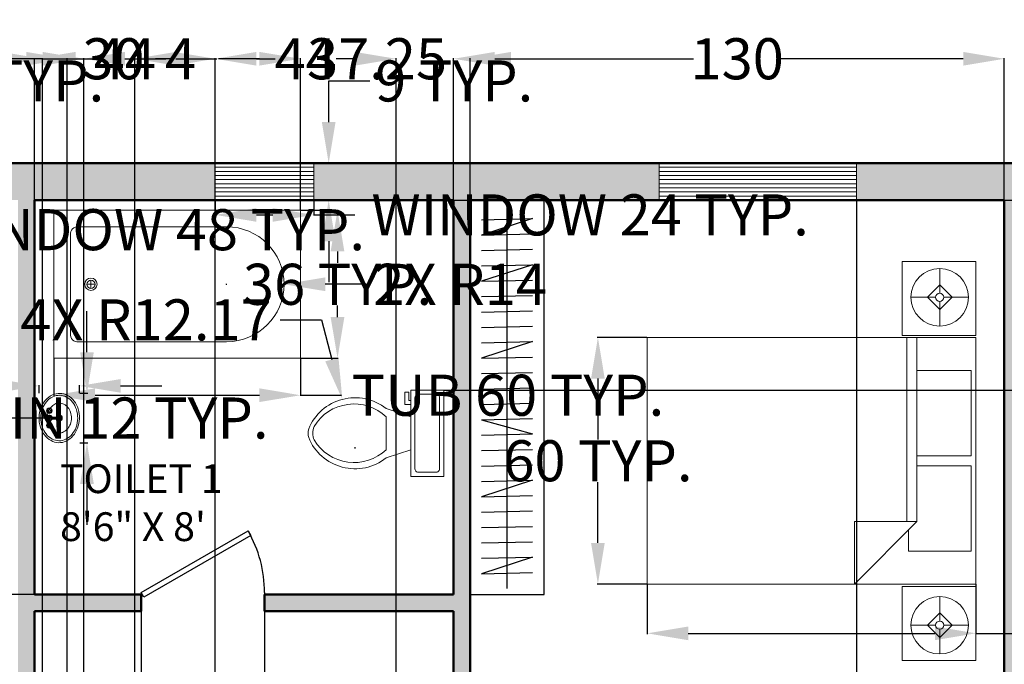
# Model space of a CAD drawing. Units: inches. Extents: x 133 to 758, y -29 to 543.
# Tile 6 of 7: x 386 to 626, y 386 to 543. Entities that reach past the tile are written whole.
import ezdxf

# ---------------------------------------------------------------- set-up
doc = ezdxf.new("R2010")
doc.units = ezdxf.units.IN
doc.header["$MEASUREMENT"] = 0
for name, color, linetype, lineweight in [('A-ANNO-DIMS', 2, 'Continuous', 18), ('A-AREA-IDEN', 7, 'Continuous', 25), ('A-FLOR-CASE', 32, 'Continuous', 25), ('A-FLOR-FIXT', 9, 'Continuous', 20), ('A-FURN', 8, 'Continuous', 18), ('A-WALL', 7, 'Continuous', 50), ('DOOR', 40, 'Continuous', 25), ('WINDOW', 151, 'Continuous', 18)]:
    doc.layers.add(name, color=color, linetype=linetype, lineweight=lineweight)
doc.layers.add('A-WALL-PATT', color=251, linetype='Continuous', lineweight=13, true_color=0x636466)
doc.styles.get("Standard").update_dxf_attribs({"font": 'arial.ttf'})
doc.dimstyles.get("Standard").update_dxf_attribs({"dimtxt": 10, "dimasz": 10, "dimexe": 0.18, "dimexo": 0.0625, "dimgap": 0.09, "dimtad": 0, "dimtih": 1, "dimtoh": 1, "dimdec": 0, "dimzin": 0, "dimdsep": 46, "dimlunit": 4, "dimtxsty": 'Standard', "dimcen": 0.09, "dimadec": 0, "dimazin": 0, "dimtfac": 1, "dimtdec": 0, "dimtofl": 0, "dimtmove": 0, "dimatfit": 3, "dimfxl": 1, "dimtolj": 1, "dimtzin": 0, "dimarcsym": 0})

# ---------------------------------------------------------------- blocks, each defined once
blk = doc.blocks.new('*U11')
for p, q in [((0, 0), (0, -6)), ((40, 0), (40, -6))]:
    blk.add_line(p, q)
blk.add_lwpolyline([(0, 0), (34.64, 20), (35.52, 18.48), (0.87, -1.52)], close=True)
blk.add_arc((0, 0), 40, 0, 30)
blk = doc.blocks.new('Bed - Queen')
for p, q in [((0, -80.00003), (0, 0)), ((0, 0), (59.99999, 0)), ((59.99999, 0), (59.99999, -80.00003)), ((7.99999, -1.2), (28.79998, -1.2)), ((7.99999, -14.4), (7.99999, -1.2)), ((28.79998, -1.2), (28.79998, -14.4)), ((31.19999, -1.2), (51.99999, -1.2)), ((31.19999, -14.4), (31.19999, -1.2)), ((51.99999, -1.2), (51.99999, -16.4)), ((0, -14.4), (44.8, -14.4)), ((59.99999, -29.6), (44.8, -14.4)), ((44.8, -14.4), (44.8, -29.6)), ((51.99999, -16.4), (46.79936, -16.4)), ((44.8, -16.8), (0, -16.8)), ((44.8, -29.6), (59.99999, -29.6)), ((59.99999, -80.00003), (0, -80.00003))]:
    blk.add_line(p, q)
blk = doc.blocks.new('Lamp - Table')
for p, q in [((0, 7), (0, 1)), ((0, 3), (-3, 0)), ((3, 0), (0, 3)), ((-1, 0), (-7, 0)), ((-3, 0), (0, -3)), ((0, -3), (3, 0)), ((1, 0), (7, 0)), ((0, -1), (0, -7))]:
    blk.add_line(p, q)
for radius in [7, 1]:
    blk.add_circle((0, 0), radius)
blk = doc.blocks.new('Bath Tub - 26 x 60 in.')
for p, q in [((8, -18), (10, -18)), ((9, -17), (9, -19))]:
    blk.add_line(p, q)
blk.add_lwpolyline([(0, -36), (0, 0), (60, 0), (60, -36)], close=True)
for points in [[(6, -4), (42, -4)], [(4, -30), (4, -6)], [(42, -32), (6, -32)]]:
    blk.add_lwpolyline(points)
for radius in [1.5, 1]:
    blk.add_circle((9, -18), radius)
for centre, radius, start, end in [((5.75, -5.75), 1.77, 81.8699, 188.1301), ((42, -18), 14, 270, 90), ((5.75, -30.25), 1.77, 171.8699, 278.1301)]:
    blk.add_arc(centre, radius, start, end)
blk = doc.blocks.new('Toilet - top')
for p, q in [((9.5, -6), (9.5, -2)), ((-10, -8.5), (-8, -8.5)), ((-10, -9.5), (-10, -8.5)), ((-7, -9.5), (-10, -9.5)), ((-8, -8.5), (-8, -8)), ((-7, -8), (-7, -9.5)), ((-4, -8), (-6, -14)), ((4, -8), (6, -14)), ((4, -14), (-4, -14))]:
    blk.add_line(p, q)
blk.add_lwpolyline([(10.5, -8), (10.5, 0), (-10.5, 0), (-10.5, -8)], close=True)
for points in [[(-9.5, -2), (-9.5, -6)], [(8.5, -1), (-8.5, -1)], [(-8.5, -7), (8.5, -7)]]:
    blk.add_lwpolyline(points)
for centre, radius, start, end in [((-8.62, -1.88), 0.884, 81.8699, 188.1301), ((8.62, -1.88), 0.884, 351.8699, 98.1301), ((-8.62, -6.12), 0.884, 171.8699, 278.1301), ((8.62, -6.12), 0.884, 261.8699, 8.1301), ((3.52, -21.58), 12.17, 141.4691, 247.9714), ((4.2, -21.82), 11.33, 136.3677, 238.9468), ((-3.52, -21.58), 12.17, 292.0284, 38.5307), ((-4.2, -21.82), 11.33, 301.053, 43.6321), ((0, -27.88), 4, 245.7318, 294.2682), ((0, -29), 4, 254.8605, 285.1395)]:
    blk.add_arc(centre, radius, start, end)
blk = doc.blocks.new('Sink - Oval top')
for p, q in [((-1, 0), (1, 0)), ((0, 1), (0, -1))]:
    blk.add_line(p, q)
for points in [[(-12.23, 0.39, 0.117634), (-11.46, -3.36, 0.104469), (-8.88, -6.8, 0.090016), (-5.08, -9.07, 0.08192), (-0.32, -10.02, 0.08192), (4.49, -9.38, 0.090016), (8.42, -7.36, 0.104469), (11.22, -4.09, 0.117634), (12.23, -0.39, 0.117634), (11.46, 3.36, 0.104469), (8.88, 6.8, 0.090016), (5.08, 9.07, 0.08192), (0.32, 10.02, 0.08192), (-4.49, 9.38, 0.090016), (-8.42, 7.36, 0.104469), (-11.22, 4.09, 0.117634)], [(-11.29, 0.16, 0.118622), (-10.52, -3.25, 0.104678), (-8.07, -6.36, 0.089562), (-4.54, -8.37, 0.081185), (-0.13, -9.15, 0.081185), (4.3, -8.49, 0.089562), (7.89, -6.58, 0.104678), (10.42, -3.55, 0.118622), (11.29, -0.16, 0.118622), (10.52, 3.25, 0.104678), (8.07, 6.36, 0.089562), (4.54, 8.37, 0.081185), (0.13, 9.15, 0.081185), (-4.3, 8.49, 0.089562), (-7.89, 6.58, 0.104678), (-10.42, 3.55, 0.118622)], [(-7.42, 0.08, 0.118283), (-6.91, -2.17, 0.104607), (-5.29, -4.21, 0.089718), (-2.97, -5.53, 0.081436), (-0.07, -6.04, 0.081436), (2.84, -5.59, 0.089718), (5.2, -4.33, 0.104607), (6.86, -2.32, 0.118283), (7.42, -0.08, 0.118283), (6.91, 2.17, 0.104607), (5.29, 4.21, 0.089718), (2.97, 5.53, 0.081436), (0.07, 6.04, 0.081436), (-2.84, 5.59, 0.089718), (-5.2, 4.33, 0.104607), (-6.86, 2.32, 0.118283)]]:
    blk.add_lwpolyline(points, format="xyb", close=True)
for radius in [1.5, 1]:
    blk.add_circle((0, 0), radius)
blk = doc.blocks.new('Faucet - Bathroom top')
for p, q in [((-4.107, 0.125), (-4.375, 0.125)), ((-3.75, 0.4788), (-3.75, 0.75)), ((-3.5, 0.482), (-3.5, 0.75)), ((-3.1461, 0.125), (-2.875, 0.125)), ((3.143, 0.125), (2.875, 0.125)), ((3.5, 0.4788), (3.5, 0.75)), ((3.75, 0.482), (3.75, 0.75)), ((4.1039, 0.125), (4.375, 0.125)), ((-4.1039, -0.125), (-4.375, -0.125)), ((-3.75, -0.4821), (-3.75, -0.75)), ((-3.5, -0.4789), (-3.5, -0.75)), ((-3.143, -0.125), (-2.875, -0.125)), ((-0.5, -0.8639), (-0.5, -4.5)), ((0.5, -4.5), (0.5, -0.8631)), ((3.1461, -0.125), (2.875, -0.125)), ((3.5, -0.4821), (3.5, -0.75)), ((3.75, -0.4789), (3.75, -0.75)), ((4.107, -0.125), (4.375, -0.125))]:
    blk.add_line(p, q)
for centre, radius in [((-3.625, 0), 1.375), ((-4.625, 0), 0.2795), ((-3.625, 0), 0.5), ((-3.625, 1), 0.2795), ((-2.625, 0), 0.2795), ((0, 0), 0.5), ((3.625, 0), 1.375), ((2.625, 0), 0.2795), ((3.625, 0), 0.5), ((3.625, 1), 0.2795), ((4.625, 0), 0.2795), ((-3.625, -1), 0.2795), ((3.625, -1), 0.2795)]:
    blk.add_circle(centre, radius)
for centre, radius, start, end in [((-3.625, 0), 1, 105.2407, 164.2093), ((-3.625, 0), 1, 16.44125, 74.07887), ((0, 0), 1.5, 289.6514, 250.3603), ((0, 0), 1, 300.3431, 239.7554), ((3.625, 0), 1, 106.12, 164.0884), ((3.625, 0), 1, 16.23422, 73.90469), ((-3.625, 0), 1, 196.2342, 253.9047), ((-3.625, 0), 1, 286.12, 344.0884), ((0, -4.5), 0.5, 180, 0), ((3.625, 0), 1, 196.4413, 254.0789), ((3.625, 0), 1, 285.2407, 344.2093)]:
    blk.add_arc(centre, radius, start, end)
blk = doc.blocks.new('WIN-48IN')
for p, q in [((0, 8), (48, 8)), ((0, 7), (48, 7)), ((0, 6), (48, 6)), ((0, 5), (48, 5)), ((0, 4), (48, 4)), ((0, 3), (48, 3)), ((0, 2), (48, 2)), ((0, 1), (48, 1)), ((0, 0), (48, 0))]:
    blk.add_line(p, q)
blk.add_lwpolyline([(48, 9), (48, 0), (0, 0), (0, 9)], close=True)
blk = doc.blocks.new('WIN-24IN')
for p, q in [((0, 8), (24, 8)), ((0, 7), (24, 7)), ((0, 6), (24, 6)), ((0, 5), (24, 5)), ((0, 4), (24, 4)), ((0, 3), (24, 3)), ((0, 2), (24, 2)), ((0, 1), (24, 1))]:
    blk.add_line(p, q)
blk.add_lwpolyline([(24, 9), (24, 0), (0, 0), (0, 9)], close=True)
blk = doc.blocks.new('WARDROBE-96X18IN')
for p, q in [((18, 96), (0, 96)), ((0, 96), (0, 0)), ((18, 0), (18, 96)), ((9, 1.47), (9, 94.4)), ((2.8, 91.24), (15.16, 91.53)), ((15.16, 91.53), (2.8, 87.49)), ((2.8, 87.49), (15.16, 87.78)), ((2.8, 83.75), (15.16, 84.04)), ((2.8, 80), (15.16, 80.29)), ((15.16, 80.29), (2.8, 76.25)), ((2.8, 76.25), (15.16, 76.54)), ((2.8, 72.51), (15.16, 72.8)), ((2.8, 68.76), (15.16, 69.05)), ((2.8, 65.01), (15.16, 65.3)), ((2.8, 61.27), (15.16, 61.56)), ((15.16, 61.56), (2.8, 57.52)), ((2.8, 57.52), (15.16, 57.81)), ((2.8, 53.77), (15.16, 54.06)), ((2.8, 50.03), (15.16, 50.32)), ((2.8, 46.28), (15.16, 46.57)), ((2.8, 42.53), (15.16, 42.82)), ((2.8, 42.53), (15.16, 39.08)), ((2.8, 38.79), (15.16, 39.08)), ((2.8, 35.04), (15.16, 35.33)), ((2.8, 31.29), (15.16, 31.58)), ((2.8, 27.55), (15.16, 27.84)), ((15.16, 27.84), (2.8, 23.8)), ((2.8, 23.8), (15.16, 24.09)), ((2.8, 20.06), (15.16, 20.35)), ((2.8, 16.31), (15.16, 16.6)), ((2.8, 12.56), (15.16, 12.85)), ((2.8, 8.82), (15.16, 9.11)), ((15.16, 9.11), (2.8, 5.07)), ((2.8, 5.07), (15.16, 5.36)), ((0, 0), (18, 0))]:
    blk.add_line(p, q)
blk = doc.blocks.new('NIGHTSTAND-18IN')
blk.add_lwpolyline([(18, 18), (18, 0), (0, 0), (0, 18)], close=True)
blk = doc.blocks.new('*D42')
at = {"layer": 'A-ANNO-DIMS', "color": 0, "lineweight": -2, "transparency": 16777216}
for p, q in [((301.75, 499.27), (301.75, 491.96)), ((349.75, 499.27), (349.75, 491.96)), ((311.75, 492.14), (339.75, 492.14)), ((349.75, 492.14), (359.75, 492.14))]:
    blk.add_line(p, q, dxfattribs=at)
at = {"layer": 'A-ANNO-DIMS', "color": 0, "transparency": 16777216}
for points in [[(311.75, 493.8), (311.75, 490.47), (301.75, 492.14)], [(339.75, 493.8), (339.75, 490.47), (349.75, 492.14)]]:
    blk.add_solid(points, dxfattribs=at)
at = {"layer": 'Defpoints', "color": 0, "transparency": 16777216}
for p in [(301.75, 499.34), (349.75, 499.34), (349.75, 492.14)]:
    blk.add_point(p, dxfattribs=at)
at = {"layer": 'A-ANNO-DIMS', "color": 0, "transparency": 16777216, "insert": (416.97, 492.14), "char_height": 10, "attachment_point": 5}
blk.add_mtext('\\A1;WINDOW 48 TYP.', dxfattribs=at)
blk = doc.blocks.new('*D43')
at = {"layer": 'A-ANNO-DIMS', "color": 0, "lineweight": -2, "transparency": 16777216}
for p, q in [((356.95, 518.34), (356.95, 528.34)), ((356.95, 528.34), (366.95, 528.34)), ((349.81, 508.34), (357.13, 508.34)), ((349.81, 499.34), (357.13, 499.34)), ((356.95, 489.34), (356.95, 479.34))]:
    blk.add_line(p, q, dxfattribs=at)
at = {"layer": 'A-ANNO-DIMS', "color": 0, "transparency": 16777216}
for points in [[(355.28, 518.34), (358.62, 518.34), (356.95, 508.34)], [(355.28, 489.34), (358.62, 489.34), (356.95, 499.34)]]:
    blk.add_solid(points, dxfattribs=at)
at = {"layer": 'Defpoints', "color": 0, "transparency": 16777216}
for p in [(349.75, 508.34), (356.95, 508.34), (349.75, 499.34)]:
    blk.add_point(p, dxfattribs=at)
at = {"layer": 'A-ANNO-DIMS', "color": 0, "transparency": 16777216, "insert": (387.49, 528.34), "char_height": 10, "attachment_point": 5}
blk.add_mtext('\\A1;9 TYP.', dxfattribs=at)
blk = doc.blocks.new('*D44')
at = {"layer": 'A-ANNO-DIMS', "color": 0, "lineweight": -2, "transparency": 16777216}
for p, q in [((538.86, 405.84), (538.86, 393.72)), ((618.86, 405.84), (618.86, 393.72)), ((548.86, 393.9), (608.86, 393.9)), ((618.86, 393.9), (628.86, 393.9))]:
    blk.add_line(p, q, dxfattribs=at)
at = {"layer": 'A-ANNO-DIMS', "color": 0, "transparency": 16777216}
for points in [[(548.86, 395.56), (548.86, 392.23), (538.86, 393.9)], [(608.86, 395.56), (608.86, 392.23), (618.86, 393.9)]]:
    blk.add_solid(points, dxfattribs=at)
at = {"layer": 'Defpoints', "color": 0, "transparency": 16777216}
for p in [(538.86, 405.9), (618.86, 405.9), (618.86, 393.9)]:
    blk.add_point(p, dxfattribs=at)
at = {"layer": 'A-ANNO-DIMS', "color": 0, "transparency": 16777216, "insert": (696.36, 393.9), "char_height": 10, "attachment_point": 5}
blk.add_mtext('\\A1;QUEEN BED 80 TYP.', dxfattribs=at)
blk = doc.blocks.new('*D45')
at = {"layer": 'A-ANNO-DIMS', "color": 0, "lineweight": -2, "transparency": 16777216}
for p, q in [((538.79, 465.9), (526.68, 465.9)), ((526.86, 455.9), (526.86, 441.09)), ((526.86, 415.9), (526.86, 430.7)), ((538.79, 405.9), (526.68, 405.9))]:
    blk.add_line(p, q, dxfattribs=at)
at = {"layer": 'A-ANNO-DIMS', "color": 0, "transparency": 16777216}
for points in [[(525.19, 455.9), (528.52, 455.9), (526.86, 465.9)], [(525.19, 415.9), (528.52, 415.9), (526.86, 405.9)]]:
    blk.add_solid(points, dxfattribs=at)
at = {"layer": 'Defpoints', "color": 0, "transparency": 16777216}
for p in [(538.86, 465.9), (526.86, 405.9), (538.86, 405.9)]:
    blk.add_point(p, dxfattribs=at)
at = {"layer": 'A-ANNO-DIMS', "color": 0, "transparency": 16777216, "insert": (526.86, 435.9), "char_height": 10, "attachment_point": 5}
blk.add_mtext('\\A1;60 TYP.', dxfattribs=at)
blk = doc.blocks.new('*D48')
at = {"layer": 'A-ANNO-DIMS', "color": 0, "lineweight": -2, "transparency": 16777216}
for p, q in [((394.5, 460.79), (394.5, 451.67)), ((454.5, 460.79), (454.5, 451.67)), ((404.5, 451.85), (444.5, 451.85)), ((454.5, 451.85), (464.5, 451.85))]:
    blk.add_line(p, q, dxfattribs=at)
at = {"layer": 'A-ANNO-DIMS', "color": 0, "transparency": 16777216}
for points in [[(404.5, 453.52), (404.5, 450.19), (394.5, 451.85)], [(444.5, 453.52), (444.5, 450.19), (454.5, 451.85)]]:
    blk.add_solid(points, dxfattribs=at)
at = {"layer": 'Defpoints', "color": 0, "transparency": 16777216}
for p in [(394.5, 460.85), (454.5, 460.85), (454.5, 451.85)]:
    blk.add_point(p, dxfattribs=at)
at = {"layer": 'A-ANNO-DIMS', "color": 0, "transparency": 16777216, "insert": (504.96, 451.85), "char_height": 10, "attachment_point": 5}
blk.add_mtext('\\A1;TUB 60 TYP.', dxfattribs=at)
blk = doc.blocks.new('*D49')
at = {"layer": 'A-ANNO-DIMS', "color": 0, "lineweight": -2, "transparency": 16777216}
for p, q in [((454.56, 496.85), (463.68, 496.85)), ((463.5, 486.85), (463.5, 484.05)), ((463.5, 470.85), (463.5, 473.65)), ((454.56, 460.85), (463.68, 460.85))]:
    blk.add_line(p, q, dxfattribs=at)
at = {"layer": 'A-ANNO-DIMS', "color": 0, "transparency": 16777216}
for points in [[(461.83, 486.85), (465.16, 486.85), (463.5, 496.85)], [(461.83, 470.85), (465.16, 470.85), (463.5, 460.85)]]:
    blk.add_solid(points, dxfattribs=at)
at = {"layer": 'Defpoints', "color": 0, "transparency": 16777216}
for p in [(454.5, 496.85), (463.5, 496.85), (454.5, 460.85)]:
    blk.add_point(p, dxfattribs=at)
at = {"layer": 'A-ANNO-DIMS', "color": 0, "transparency": 16777216, "insert": (463.5, 478.85), "char_height": 10, "attachment_point": 5}
blk.add_mtext('\\A1;36 TYP.', dxfattribs=at)
blk = doc.blocks.new('*D52')
at = {"layer": 'A-ANNO-DIMS', "color": 0, "lineweight": -2, "transparency": 16777216}
for p, q in [((402.53, 462.32), (402.53, 472.32)), ((400.79, 452.32), (402.71, 452.32)), ((400.79, 440.28), (402.71, 440.28)), ((402.53, 430.28), (402.53, 420.28))]:
    blk.add_line(p, q, dxfattribs=at)
at = {"layer": 'A-ANNO-DIMS', "color": 0, "transparency": 16777216}
for points in [[(400.87, 462.32), (404.2, 462.32), (402.53, 452.32)], [(400.87, 430.28), (404.2, 430.28), (402.53, 440.28)]]:
    blk.add_solid(points, dxfattribs=at)
at = {"layer": 'Defpoints', "color": 0, "transparency": 16777216}
for p in [(400.73, 452.32), (402.53, 452.32), (400.73, 440.28)]:
    blk.add_point(p, dxfattribs=at)
at = {"layer": 'A-ANNO-DIMS', "color": 0, "transparency": 16777216, "insert": (402.53, 446.3), "char_height": 10, "attachment_point": 5}
blk.add_mtext('\\A1;BASIN 12 TYP.', dxfattribs=at)
blk = doc.blocks.new('*D53')
at = {"layer": 'A-ANNO-DIMS', "color": 0, "lineweight": -2, "transparency": 16777216}
for p, q in [((380.86, 454.12), (370.86, 454.12)), ((390.86, 452.38), (390.86, 454.3)), ((400.73, 452.38), (400.73, 454.3)), ((410.73, 454.12), (420.73, 454.12))]:
    blk.add_line(p, q, dxfattribs=at)
at = {"layer": 'A-ANNO-DIMS', "color": 0, "transparency": 16777216}
for points in [[(380.86, 455.79), (380.86, 452.46), (390.86, 454.12)], [(410.73, 455.79), (410.73, 452.46), (400.73, 454.12)]]:
    blk.add_solid(points, dxfattribs=at)
at = {"layer": 'Defpoints', "color": 0, "transparency": 16777216}
for p in [(390.86, 454.12), (390.86, 452.32), (400.73, 452.32)]:
    blk.add_point(p, dxfattribs=at)
at = {"layer": 'A-ANNO-DIMS', "color": 0, "transparency": 16777216, "insert": (346.9, 454.12), "char_height": 10, "attachment_point": 5}
blk.add_mtext('\\A1;10 TYP.', dxfattribs=at)
blk = doc.blocks.new('*D56')
at = {"layer": 'A-ANNO-DIMS', "color": 0, "lineweight": -2, "transparency": 16777216}
for p, q in [((433.75, 499.27), (433.75, 495.56)), ((457.75, 499.27), (457.75, 495.56)), ((443.75, 495.74), (447.75, 495.74)), ((457.75, 495.74), (467.75, 495.74))]:
    blk.add_line(p, q, dxfattribs=at)
at = {"layer": 'A-ANNO-DIMS', "color": 0, "transparency": 16777216}
for points in [[(443.75, 497.4), (443.75, 494.07), (433.75, 495.74)], [(447.75, 497.4), (447.75, 494.07), (457.75, 495.74)]]:
    blk.add_solid(points, dxfattribs=at)
at = {"layer": 'Defpoints', "color": 0, "transparency": 16777216}
for p in [(433.75, 499.34), (457.75, 499.34), (457.75, 495.74)]:
    blk.add_point(p, dxfattribs=at)
at = {"layer": 'A-ANNO-DIMS', "color": 0, "transparency": 16777216, "insert": (524.97, 495.74), "char_height": 10, "attachment_point": 5}
blk.add_mtext('\\A1;WINDOW 24 TYP.', dxfattribs=at)
blk = doc.blocks.new('*D57')
at = {"layer": 'A-ANNO-DIMS', "color": 0, "lineweight": -2, "transparency": 16777216}
for p, q in [((461.35, 518.34), (461.35, 528.34)), ((461.35, 528.34), (471.35, 528.34)), ((457.81, 508.34), (461.53, 508.34)), ((457.81, 499.34), (461.53, 499.34)), ((461.35, 489.34), (461.35, 479.34))]:
    blk.add_line(p, q, dxfattribs=at)
at = {"layer": 'A-ANNO-DIMS', "color": 0, "transparency": 16777216}
for points in [[(459.68, 518.34), (463.02, 518.34), (461.35, 508.34)], [(459.68, 489.34), (463.02, 489.34), (461.35, 499.34)]]:
    blk.add_solid(points, dxfattribs=at)
at = {"layer": 'Defpoints', "color": 0, "transparency": 16777216}
for p in [(457.75, 508.34), (461.35, 508.34), (457.75, 499.34)]:
    blk.add_point(p, dxfattribs=at)
at = {"layer": 'A-ANNO-DIMS', "color": 0, "transparency": 16777216, "insert": (491.89, 528.34), "char_height": 10, "attachment_point": 5}
blk.add_mtext('\\A1;9 TYP.', dxfattribs=at)
blk = doc.blocks.new('*D74')
at = {"layer": 'A-ANNO-DIMS', "color": 0, "lineweight": -2, "transparency": 16777216}
for p, q in [((495.75, 499.4), (495.75, 533.92)), ((505.75, 533.74), (550.1, 533.74)), ((615.75, 533.74), (571.4, 533.74)), ((625.75, 499.4), (625.75, 533.92))]:
    blk.add_line(p, q, dxfattribs=at)
at = {"layer": 'A-ANNO-DIMS', "color": 0, "transparency": 16777216}
for points in [[(505.75, 535.4), (505.75, 532.07), (495.75, 533.74)], [(615.75, 535.4), (615.75, 532.07), (625.75, 533.74)]]:
    blk.add_solid(points, dxfattribs=at)
at = {"layer": 'Defpoints', "color": 0, "transparency": 16777216}
for p in [(625.75, 533.74), (495.75, 499.34), (625.75, 499.34)]:
    blk.add_point(p, dxfattribs=at)
at = {"layer": 'A-ANNO-DIMS', "color": 0, "transparency": 16777216, "insert": (560.75, 533.74), "char_height": 10, "attachment_point": 5}
blk.add_mtext('\\A1;130', dxfattribs=at)
blk = doc.blocks.new('*D78')
at = {"layer": 'A-ANNO-DIMS', "color": 0, "lineweight": -2, "transparency": 16777216}
for p, q in [((361.75, 167.4), (361.75, 533.92)), ((371.75, 533.74), (381.75, 533.74)), ((391.75, 167.4), (391.75, 533.92)), ((391.75, 533.74), (401.75, 533.74))]:
    blk.add_line(p, q, dxfattribs=at)
at = {"layer": 'A-ANNO-DIMS', "color": 0, "transparency": 16777216}
for points in [[(371.75, 535.4), (371.75, 532.07), (361.75, 533.74)], [(381.75, 535.4), (381.75, 532.07), (391.75, 533.74)]]:
    blk.add_solid(points, dxfattribs=at)
at = {"layer": 'Defpoints', "color": 0, "transparency": 16777216}
for p in [(391.75, 533.74), (361.75, 167.34), (391.75, 167.34)]:
    blk.add_point(p, dxfattribs=at)
at = {"layer": 'A-ANNO-DIMS', "color": 0, "transparency": 16777216, "insert": (408.98, 533.74), "char_height": 10, "attachment_point": 5}
blk.add_mtext('\\A1;30', dxfattribs=at)
blk = doc.blocks.new('*D80')
at = {"layer": 'A-ANNO-DIMS', "color": 0, "lineweight": -2, "transparency": 16777216}
for p, q in [((389.75, 499.4), (389.75, 533.92)), ((399.75, 533.74), (404.32, 533.74)), ((423.75, 533.74), (419.18, 533.74)), ((433.75, 499.4), (433.75, 533.92))]:
    blk.add_line(p, q, dxfattribs=at)
at = {"layer": 'A-ANNO-DIMS', "color": 0, "transparency": 16777216}
for points in [[(399.75, 535.4), (399.75, 532.07), (389.75, 533.74)], [(423.75, 535.4), (423.75, 532.07), (433.75, 533.74)]]:
    blk.add_solid(points, dxfattribs=at)
at = {"layer": 'Defpoints', "color": 0, "transparency": 16777216}
for p in [(433.75, 533.74), (389.75, 499.34), (433.75, 499.34)]:
    blk.add_point(p, dxfattribs=at)
at = {"layer": 'A-ANNO-DIMS', "color": 0, "transparency": 16777216, "insert": (411.75, 533.74), "char_height": 10, "attachment_point": 5}
blk.add_mtext('\\A1;44', dxfattribs=at)
blk = doc.blocks.new('*D81')
at = {"layer": 'A-ANNO-DIMS', "color": 0, "lineweight": -2, "transparency": 16777216}
for p, q in [((589.75, 499.27), (589.75, -22.24)), ((625.75, 499.27), (625.75, -22.24)), ((599.75, -22.06), (600.5, -22.06)), ((615.75, -22.06), (615, -22.06))]:
    blk.add_line(p, q, dxfattribs=at)
at = {"layer": 'A-ANNO-DIMS', "color": 0, "transparency": 16777216}
for points in [[(599.75, -20.4), (599.75, -23.73), (589.75, -22.06)], [(615.75, -20.4), (615.75, -23.73), (625.75, -22.06)]]:
    blk.add_solid(points, dxfattribs=at)
at = {"layer": 'Defpoints', "color": 0, "transparency": 16777216}
for p in [(589.75, 499.34), (625.75, 499.34), (625.75, -22.06)]:
    blk.add_point(p, dxfattribs=at)
at = {"layer": 'A-ANNO-DIMS', "color": 0, "transparency": 16777216, "insert": (607.75, -22.06), "char_height": 10, "attachment_point": 5}
blk.add_mtext('\\A1;36', dxfattribs=at)
blk = doc.blocks.new('*D85')
at = {"layer": 'A-ANNO-DIMS', "color": 0, "lineweight": -2, "transparency": 16777216}
for p, q in [((389.75, 399.27), (389.75, -22.24)), ((415.75, 399.27), (415.75, -22.24)), ((389.75, -22.06), (379.75, -22.06)), ((405.75, -22.06), (399.75, -22.06))]:
    blk.add_line(p, q, dxfattribs=at)
at = {"layer": 'A-ANNO-DIMS', "color": 0, "transparency": 16777216}
for points in [[(399.75, -20.4), (399.75, -23.73), (389.75, -22.06)], [(405.75, -20.4), (405.75, -23.73), (415.75, -22.06)]]:
    blk.add_solid(points, dxfattribs=at)
at = {"layer": 'Defpoints', "color": 0, "transparency": 16777216}
for p in [(389.75, 399.34), (415.75, 399.34), (389.75, -22.06)]:
    blk.add_point(p, dxfattribs=at)
at = {"layer": 'A-ANNO-DIMS', "color": 0, "transparency": 16777216, "insert": (372.42, -22.06), "char_height": 10, "attachment_point": 5}
blk.add_mtext('\\A1;26', dxfattribs=at)
blk = doc.blocks.new('*D89')
at = {"layer": 'A-ANNO-DIMS', "color": 0, "lineweight": -2, "transparency": 16777216}
for p, q in [((387.75, 533.74), (377.75, 533.74)), ((397.75, 163.4), (397.75, 533.92)), ((401.75, 163.4), (401.75, 533.92)), ((411.75, 533.74), (421.75, 533.74))]:
    blk.add_line(p, q, dxfattribs=at)
at = {"layer": 'A-ANNO-DIMS', "color": 0, "transparency": 16777216}
for points in [[(387.75, 535.4), (387.75, 532.07), (397.75, 533.74)], [(411.75, 535.4), (411.75, 532.07), (401.75, 533.74)]]:
    blk.add_solid(points, dxfattribs=at)
at = {"layer": 'Defpoints', "color": 0, "transparency": 16777216}
for p in [(401.75, 533.74), (397.75, 163.34), (401.75, 163.34)]:
    blk.add_point(p, dxfattribs=at)
at = {"layer": 'A-ANNO-DIMS', "color": 0, "transparency": 16777216, "insert": (425.3, 533.74), "char_height": 10, "attachment_point": 5}
blk.add_mtext('\\A1;4', dxfattribs=at)
blk = doc.blocks.new('*D90')
at = {"layer": 'A-ANNO-DIMS', "color": 0, "lineweight": -2, "transparency": 16777216}
for p, q in [((433.75, 167.4), (433.75, 533.92)), ((443.75, 533.74), (448.32, 533.74)), ((467.75, 533.74), (463.18, 533.74)), ((477.75, 163.4), (477.75, 533.92))]:
    blk.add_line(p, q, dxfattribs=at)
at = {"layer": 'A-ANNO-DIMS', "color": 0, "transparency": 16777216}
for points in [[(443.75, 535.4), (443.75, 532.07), (433.75, 533.74)], [(467.75, 535.4), (467.75, 532.07), (477.75, 533.74)]]:
    blk.add_solid(points, dxfattribs=at)
at = {"layer": 'Defpoints', "color": 0, "transparency": 16777216}
for p in [(477.75, 533.74), (433.75, 167.34), (477.75, 163.34)]:
    blk.add_point(p, dxfattribs=at)
at = {"layer": 'A-ANNO-DIMS', "color": 0, "transparency": 16777216, "insert": (455.75, 533.74), "char_height": 10, "attachment_point": 5}
blk.add_mtext('\\A1;44', dxfattribs=at)
blk = doc.blocks.new('*D91')
at = {"layer": 'A-ANNO-DIMS', "color": 0, "lineweight": -2, "transparency": 16777216}
for p, q in [((415.75, 399.27), (415.75, -22.24)), ((445.75, 399.27), (445.75, -22.24)), ((425.75, -22.06), (435.75, -22.06)), ((445.75, -22.06), (455.75, -22.06))]:
    blk.add_line(p, q, dxfattribs=at)
at = {"layer": 'A-ANNO-DIMS', "color": 0, "transparency": 16777216}
for points in [[(425.75, -20.4), (425.75, -23.73), (415.75, -22.06)], [(435.75, -20.4), (435.75, -23.73), (445.75, -22.06)]]:
    blk.add_solid(points, dxfattribs=at)
at = {"layer": 'Defpoints', "color": 0, "transparency": 16777216}
for p in [(415.75, 399.34), (445.75, 399.34), (445.75, -22.06)]:
    blk.add_point(p, dxfattribs=at)
at = {"layer": 'A-ANNO-DIMS', "color": 0, "transparency": 16777216, "insert": (462.98, -22.06), "char_height": 10, "attachment_point": 5}
blk.add_mtext('\\A1;30', dxfattribs=at)
blk = doc.blocks.new('*D92')
at = {"layer": 'A-ANNO-DIMS', "color": 0, "lineweight": -2, "transparency": 16777216}
for p, q in [((395.73, 446.3), (231.17, 446.3)), ((231.35, 436.3), (231.35, 430.01)), ((231.35, 413.34), (231.35, 419.62)), ((389.69, 403.34), (231.17, 403.34))]:
    blk.add_line(p, q, dxfattribs=at)
at = {"layer": 'A-ANNO-DIMS', "color": 0, "transparency": 16777216}
for points in [[(229.68, 436.3), (233.02, 436.3), (231.35, 446.3)], [(229.68, 413.34), (233.02, 413.34), (231.35, 403.34)]]:
    blk.add_solid(points, dxfattribs=at)
at = {"layer": 'Defpoints', "color": 0, "transparency": 16777216}
for p in [(395.79, 446.3), (231.35, 403.34), (389.75, 403.34)]:
    blk.add_point(p, dxfattribs=at)
at = {"layer": 'A-ANNO-DIMS', "color": 0, "transparency": 16777216, "insert": (231.35, 424.82), "char_height": 10, "attachment_point": 5}
blk.add_mtext('\\A1;42.965', dxfattribs=at)
blk = doc.blocks.new('*D97')
at = {"layer": 'A-ANNO-DIMS', "color": 0, "lineweight": -2, "transparency": 16777216}
for p, q in [((444.5, 533.74), (434.5, 533.74)), ((454.5, 496.92), (454.5, 533.92)), ((491.75, 499.4), (491.75, 533.92)), ((501.75, 533.74), (511.75, 533.74))]:
    blk.add_line(p, q, dxfattribs=at)
at = {"layer": 'A-ANNO-DIMS', "color": 0, "transparency": 16777216}
for points in [[(444.5, 535.4), (444.5, 532.07), (454.5, 533.74)], [(501.75, 535.4), (501.75, 532.07), (491.75, 533.74)]]:
    blk.add_solid(points, dxfattribs=at)
at = {"layer": 'Defpoints', "color": 0, "transparency": 16777216}
for p in [(491.75, 533.74), (491.75, 499.34), (454.5, 496.85)]:
    blk.add_point(p, dxfattribs=at)
at = {"layer": 'A-ANNO-DIMS', "color": 0, "transparency": 16777216, "insert": (473.12, 533.74), "char_height": 10, "attachment_point": 5}
blk.add_mtext('\\A1;37.25', dxfattribs=at)
blk = doc.blocks.new('*D98')
at = {"layer": 'A-ANNO-DIMS', "color": 0, "lineweight": -2, "transparency": 16777216}
for p, q in [((491.81, 499.34), (660.33, 499.34)), ((660.15, 489.34), (660.15, 481.42)), ((660.15, 463.1), (660.15, 471.02)), ((489.4, 453.1), (660.33, 453.1))]:
    blk.add_line(p, q, dxfattribs=at)
at = {"layer": 'A-ANNO-DIMS', "color": 0, "transparency": 16777216}
for points in [[(658.48, 489.34), (661.82, 489.34), (660.15, 499.34)], [(658.48, 463.1), (661.82, 463.1), (660.15, 453.1)]]:
    blk.add_solid(points, dxfattribs=at)
at = {"layer": 'Defpoints', "color": 0, "transparency": 16777216}
for p in [(491.75, 499.34), (660.15, 499.34), (489.34, 453.1)]:
    blk.add_point(p, dxfattribs=at)
at = {"layer": 'A-ANNO-DIMS', "color": 0, "transparency": 16777216, "insert": (660.15, 476.22), "char_height": 10, "attachment_point": 5}
blk.add_mtext('\\A1;46.235', dxfattribs=at)
blk = doc.blocks.new('*D99')
at = {"layer": 'A-ANNO-DIMS', "color": 0, "lineweight": -2, "transparency": 16777216}
for p, q in [((391.75, 533.74), (381.75, 533.74)), ((401.75, 19.4), (401.75, 533.92)), ((414.17, 21.95), (414.17, 533.92)), ((424.17, 533.74), (434.17, 533.74))]:
    blk.add_line(p, q, dxfattribs=at)
at = {"layer": 'A-ANNO-DIMS', "color": 0, "transparency": 16777216}
for points in [[(391.75, 535.4), (391.75, 532.07), (401.75, 533.74)], [(424.17, 535.4), (424.17, 532.07), (414.17, 533.74)]]:
    blk.add_solid(points, dxfattribs=at)
at = {"layer": 'Defpoints', "color": 0, "transparency": 16777216}
for p in [(401.75, 533.74), (414.17, 21.89), (401.75, 19.34)]:
    blk.add_point(p, dxfattribs=at)
at = {"layer": 'A-ANNO-DIMS', "color": 0, "transparency": 16777216, "insert": (361.37, 533.74), "char_height": 10, "attachment_point": 5}
blk.add_mtext('\\A1;12.417', dxfattribs=at)
blk = doc.blocks.new('*D100')
at = {"layer": 'A-ANNO-DIMS', "color": 0, "lineweight": -2, "transparency": 16777216}
for p, q in [((436.41, 478.85), (436.59, 478.85)), ((436.5, 478.76), (436.5, 478.94)), ((470.5, 478.85), (460.5, 478.85))]:
    blk.add_line(p, q, dxfattribs=at)
at = {"layer": 'A-ANNO-DIMS', "color": 0, "transparency": 16777216}
blk.add_solid([(460.5, 480.52), (460.5, 477.19), (450.5, 478.85)], dxfattribs=at)
at = {"layer": 'Defpoints', "color": 0, "transparency": 16777216}
for p in [(436.5, 478.85), (450.5, 478.85)]:
    blk.add_point(p, dxfattribs=at)
at = {"layer": 'A-ANNO-DIMS', "color": 0, "transparency": 16777216, "insert": (493.34, 478.85), "char_height": 10, "attachment_point": 5}
blk.add_mtext('\\A1;2X R14', dxfattribs=at)
blk = doc.blocks.new('*D101')
at = {"layer": 'A-ANNO-DIMS', "color": 0, "lineweight": -2, "transparency": 16777216}
for p, q in [((449.58, 470.19), (459.58, 470.19)), ((459.58, 470.19), (462.13, 460.52)), ((467.67, 439.08), (467.85, 439.08)), ((467.76, 438.99), (467.76, 439.17))]:
    blk.add_line(p, q, dxfattribs=at)
at = {"layer": 'A-ANNO-DIMS', "color": 0, "transparency": 16777216}
blk.add_solid([(463.74, 460.95), (460.51, 460.1), (464.67, 450.85)], dxfattribs=at)
at = {"layer": 'Defpoints', "color": 0, "transparency": 16777216}
for p in [(464.67, 450.85), (467.76, 439.08)]:
    blk.add_point(p, dxfattribs=at)
at = {"layer": 'A-ANNO-DIMS', "color": 0, "transparency": 16777216, "insert": (416.89, 470.19), "char_height": 10, "attachment_point": 5}
blk.add_mtext('\\A1;4X R12.17', dxfattribs=at)

msp = doc.modelspace()

# ---------------------------------------------------------------- hatches: boundary and pattern name
at = {"layer": 'A-WALL-PATT'}
h = msp.add_hatch(color=256, dxfattribs=at)
h.dxf.hatch_style = 1
h.paths.add_polyline_path([(433.7501, 508.336), (349.7501, 508.336), (349.7501, 499.336), (385.7501, 499.336), (385.7501, 403.336), (385.7501, 355.336), (379.7501, 355.336), (379.7501, 351.336), (389.7501, 351.336), (389.7501, 399.336), (415.7501, 399.336), (415.7501, 403.336), (389.7501, 403.336), (389.7501, 499.336), (433.7501, 499.336)])
h.paths.add_polyline_path([(541.7501, 508.336), (457.7501, 508.336), (457.7501, 499.336), (491.7501, 499.336), (491.7501, 403.336), (445.7501, 403.336), (445.7501, 399.336), (491.7501, 399.336), (491.7501, 351.336), (495.7501, 351.336), (495.7501, 399.336), (495.7501, 499.336), (513.7501, 499.336), (541.7501, 499.336)])
h.paths.add_polyline_path([(634.7501, 508.336), (589.7501, 508.336), (589.7501, 499.336), (625.7501, 499.336), (625.7501, 355.336), (525.7501, 355.336), (525.7501, 351.336), (525.7501, 307.336), (529.7501, 307.336), (529.7501, 351.336), (625.7501, 351.336), (625.7501, 283.336), (634.7501, 283.336)])
h.paths.add_polyline_path([(301.7501, 508.336), (256.7501, 508.336), (256.7501, 283.336), (265.7501, 283.336), (265.7501, 351.336), (349.7501, 351.336), (349.7501, 355.336), (265.7501, 355.336), (265.7501, 499.336), (301.7501, 499.336)])
h.paths.add_polyline_path([(361.7501, 167.336), (265.7501, 167.336), (265.7501, 235.336), (256.7501, 235.336), (256.7501, 10.336), (309.4362, 10.336), (309.4362, 19.336), (265.7501, 19.336), (265.7501, 163.336), (283.7501, 163.336), (361.7501, 163.336)])

# ---------------------------------------------------------------- linework, layer by layer
at = {"layer": 'A-WALL'}
for p, q in [((389.7501, 499.336), (491.7501, 499.336)), ((389.7501, 403.336), (389.7501, 499.336)), ((491.7501, 499.336), (491.7501, 403.336)), ((495.7501, 499.336), (625.7501, 499.336)), ((495.7501, 499.336), (495.7501, 399.336)), ((625.7501, 499.336), (625.7501, 355.336)), ((389.7501, 403.336), (415.7501, 403.336)), ((415.7501, 403.336), (415.7501, 399.336)), ((445.7501, 403.336), (445.7501, 399.336)), ((445.7501, 403.336), (491.7501, 403.336)), ((389.7501, 351.336), (389.7501, 399.336)), ((389.7501, 399.336), (415.7501, 399.336)), ((445.7501, 399.336), (491.7501, 399.336)), ((491.7501, 399.336), (491.7501, 351.336)), ((495.7501, 399.336), (495.7501, 351.336))]:
    msp.add_line(p, q, dxfattribs=at)
msp.add_lwpolyline([(505.7501, 10.336), (256.7501, 10.336), (256.7501, 508.336), (634.7501, 508.336), (634.7501, 10.336), (601.3503, 10.336)], dxfattribs=at)

# ---------------------------------------------------------------- block references
at = {"layer": 'A-FLOR-CASE'}
msp.add_blockref('WARDROBE-96X18IN', (495.75, 403.336), dxfattribs=at)
at = {"layer": 'A-FLOR-FIXT'}
msp.add_blockref('Bath Tub - 26 x 60 in.', (394.4968, 496.854), dxfattribs=at)
at = {"layer": 'A-FLOR-FIXT', "rotation": 270}
msp.add_blockref('Toilet - top', (489.3397, 442.6011), dxfattribs=at)
at = {"layer": 'A-FLOR-FIXT', "xscale": 0.4902491559291568, "yscale": 0.4902491559291568, "zscale": 0.4902491559291568, "rotation": 90}
for name, p in [('Sink - Oval top', (395.7917, 446.3011)), ('Faucet - Bathroom top', (393.3605, 446.3006))]:
    msp.add_blockref(name, p, dxfattribs=at)
at = {"layer": 'A-FURN'}
for p in [(600.857, 466.3898), (600.857, 387.29)]:
    msp.add_blockref('NIGHTSTAND-18IN', p, dxfattribs=at)
at = {"layer": 'A-FURN', "rotation": 270}
for name, p in [('Lamp - Table', (610.0308, 475.6867)), ('Bed - Queen', (618.8575, 465.8976)), ('Lamp - Table', (610.0392, 395.8808))]:
    msp.add_blockref(name, p, dxfattribs=at)
at = {"layer": 'DOOR', "xscale": 0.75, "yscale": 0.75, "zscale": 0.75}
msp.add_blockref('*U11', (415.7501, 403.836), dxfattribs=at)
at = {"layer": 'WINDOW'}
for name, p in [('WIN-24IN', (433.75, 499.336)), ('WIN-48IN', (541.75, 499.336))]:
    msp.add_blockref(name, p, dxfattribs=at)

# ---------------------------------------------------------------- texts
at = {"layer": 'A-AREA-IDEN', "insert": (395.9785, 435.0302), "char_height": 7, "attachment_point": 1}
msp.add_mtext_dynamic_manual_height_columns('TOILET 1 \\P8\'6" X 8\'', width=89.914564, gutter_width=1, heights=[0], dxfattribs=at)

# ---------------------------------------------------------------- dimensions: what is measured, and where the dimension line sits
at = {"layer": 'A-ANNO-DIMS'}
for base, p1, p2, angle, text, picture, middle in [((356.9501, 508.336), (349.7501, 499.336), (349.7501, 508.336), 90, '<> TYP.', '*D43', (387.4937, 528.336)), ((461.3501, 508.336), (457.7501, 499.336), (457.7501, 508.336), 90, '<> TYP.', '*D57', (491.8937, 528.336)), ((463.4968, 496.854), (454.4968, 460.854), (454.4968, 496.854), 90, '<> TYP.', '*D49', (463.4968, 478.854)), ((402.533, 452.3191), (400.7276, 440.283), (400.7276, 452.3191), 90, 'BASIN <> TYP.', '*D52', (402.533, 446.3011)), ((390.8557, 454.1245), (400.7276, 452.3191), (390.8557, 452.3191), 180, '<> TYP.', '*D53', (346.898, 454.1245)), ((526.8574, 405.8976), (538.8574, 465.8976), (538.8574, 405.8976), 270, '<> TYP.', '*D45', (526.8574, 435.8976))]:
    dim = msp.add_linear_dim(base=base, p1=p1, p2=p2, angle=angle, text=text, dimstyle='Standard', override={"dimdec": 0, "dimlfac": 1, "dimrnd": 0, "dimzin": 0, "dimdsep": 46, "dimlunit": 2}, dxfattribs=at)
    dim.commit()
    dim.dimension.update_dxf_attribs({"geometry": picture, "text_midpoint": middle})
for base, p1, p2, override, picture, middle in [((401.75012, 533.73604), (414.16755, 21.88596), (401.75012, 19.33604), {"dimdec": 3, "dimlfac": 1, "dimrnd": 0, "dimzin": 0, "dimdsep": 46, "dimlunit": 2}, '*D99', (361.37362, 533.73604)), ((391.7501, 533.736), (361.7501, 167.336), (391.7501, 167.336), {"dimdec": 0, "dimlfac": 1, "dimrnd": 0, "dimzin": 0, "dimdsep": 46, "dimlunit": 2}, '*D78', (408.982, 533.736)), ((401.7501, 533.736), (397.7501, 163.336), (401.7501, 163.336), {"dimdec": 0, "dimlfac": 1, "dimrnd": 0, "dimzin": 0, "dimdsep": 46, "dimlunit": 2}, '*D89', (425.2985, 533.736)), ((433.7501, 533.736), (389.7501, 499.336), (433.7501, 499.336), {"dimdec": 0, "dimlfac": 1, "dimrnd": 0, "dimzin": 0, "dimdsep": 46, "dimlunit": 2}, '*D80', (411.7501, 533.736)), ((477.7501, 533.736), (433.7501, 167.336), (477.7501, 163.336), {"dimdec": 0, "dimlfac": 1, "dimrnd": 0, "dimzin": 0, "dimdsep": 46, "dimlunit": 2}, '*D90', (455.7501, 533.736)), ((491.7501, 533.736), (454.4968, 496.854), (491.7501, 499.336), {"dimdec": 2, "dimlfac": 1, "dimrnd": 0, "dimzin": 0, "dimdsep": 46, "dimlunit": 2}, '*D97', (473.1235, 533.736)), ((625.7501, 533.736), (495.7501, 499.336), (625.7501, 499.336), {"dimdec": 0, "dimlfac": 1, "dimrnd": 0, "dimzin": 0, "dimdsep": 46, "dimlunit": 2}, '*D74', (560.7501, 533.736)), ((625.7501, -22.064), (589.7501, 499.336), (625.7501, 499.336), {"dimdec": 0, "dimlfac": 1, "dimrnd": 0, "dimzin": 0, "dimdsep": 46, "dimlunit": 2}, '*D81', (607.7501, -22.064)), ((389.7501, -22.064), (415.7501, 399.336), (389.7501, 399.336), {"dimdec": 0, "dimlfac": 1, "dimrnd": 0, "dimzin": 0, "dimdsep": 46, "dimlunit": 2}, '*D85', (372.4159, -22.064)), ((445.7501, -22.064), (415.7501, 399.336), (445.7501, 399.336), {"dimdec": 0, "dimlfac": 1, "dimrnd": 0, "dimzin": 0, "dimdsep": 46, "dimlunit": 2}, '*D91', (462.982, -22.064))]:
    dim = msp.add_linear_dim(base=base, p1=p1, p2=p2, dimstyle='Standard', override=override, dxfattribs=at)
    dim.commit()
    dim.dimension.update_dxf_attribs({"geometry": picture, "text_midpoint": middle})
for base, p1, p2, text, picture, middle in [((457.7501, 495.736), (433.7501, 499.336), (457.7501, 499.336), 'WINDOW <> TYP.', '*D56', (524.9718, 495.736)), ((349.7501, 492.136), (301.7501, 499.336), (349.7501, 499.336), 'WINDOW <> TYP.', '*D42', (416.9718, 492.136)), ((454.4968, 451.854), (394.4968, 460.854), (454.4968, 460.854), 'TUB <> TYP.', '*D48', (504.962, 451.854)), ((618.8575, 393.8976), (538.8574, 405.8976), (618.8575, 405.8976), 'QUEEN BED <> TYP.', '*D44', (696.3588, 393.8976))]:
    dim = msp.add_linear_dim(base=base, p1=p1, p2=p2, text=text, dimstyle='Standard', override={"dimdec": 0, "dimlfac": 1, "dimrnd": 0, "dimzin": 0, "dimdsep": 46, "dimlunit": 2}, dxfattribs=at)
    dim.commit()
    dim.dimension.update_dxf_attribs({"geometry": picture, "text_midpoint": middle})
for base, p1, p2, picture, middle in [((660.1501, 499.336), (489.3397, 453.1011), (491.7501, 499.336), '*D98', (660.1501, 476.2186)), ((231.3501, 403.336), (395.7917, 446.3011), (389.7501, 403.336), '*D92', (231.3501, 424.8186))]:
    dim = msp.add_linear_dim(base=base, p1=p1, p2=p2, angle=90, dimstyle='Standard', override={"dimdec": 3, "dimlfac": 1, "dimrnd": 0, "dimzin": 0, "dimdsep": 46, "dimlunit": 2}, dxfattribs=at)
    dim.commit()
    dim.dimension.update_dxf_attribs({"geometry": picture, "text_midpoint": middle})
for center, mpoint, text, override, picture, middle in [((436.4968, 478.854), (450.4968, 478.854), '2X <>', {"dimdec": 0, "dimlfac": 1, "dimrnd": 0, "dimzin": 0, "dimdsep": 46, "dimlunit": 2}, '*D100', (493.3426, 478.8541)), ((467.7592, 439.0815), (464.667, 450.8511), '4X <>', {"dimdec": 2, "dimlfac": 1, "dimrnd": 0, "dimzin": 0, "dimdsep": 46, "dimlunit": 2}, '*D101', (416.8926, 470.1947))]:
    dim = msp.add_radius_dim(center=center, mpoint=mpoint, text=text, dimstyle='Standard', override=override, dxfattribs=at)
    dim.commit()
    dim.dimension.update_dxf_attribs({"geometry": picture, "text_midpoint": middle})

doc.saveas('drawing.dxf')
